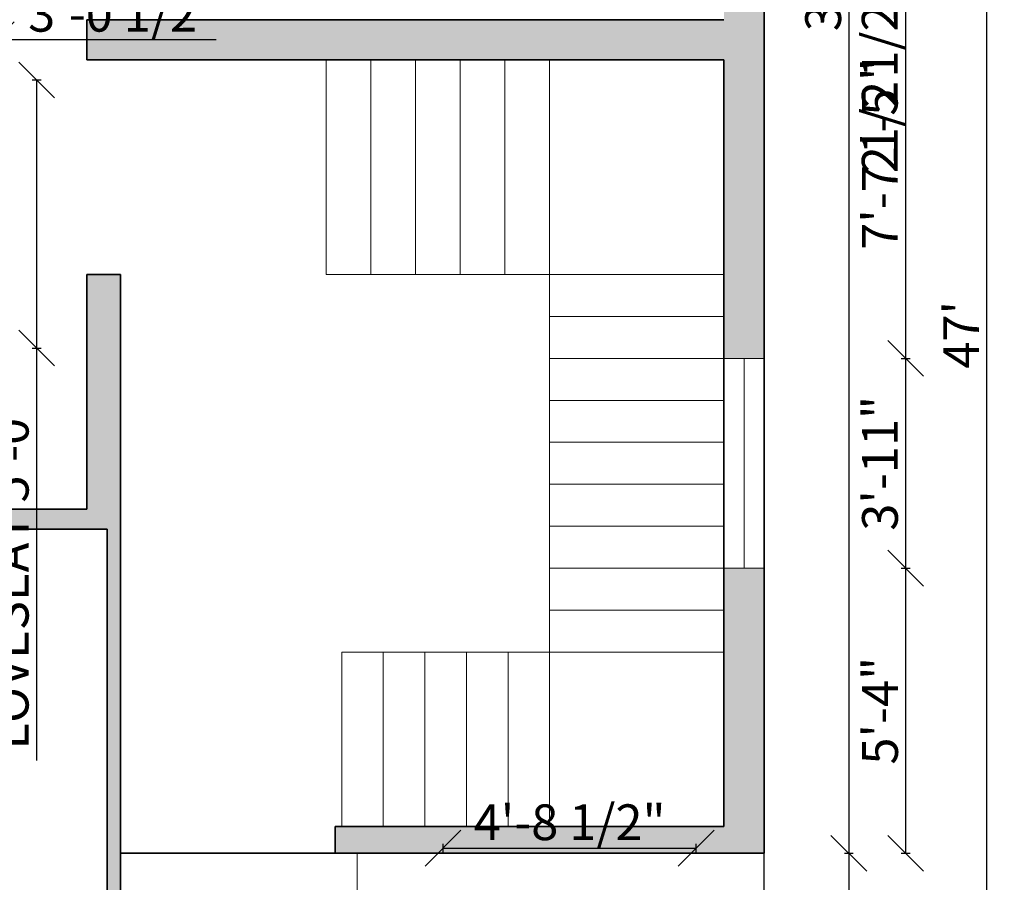
# Model space of a CAD drawing. Units: inches. Extents: x 2561 to 3163, y 493 to 1211.
# Tile 6 of 8: x 2943 to 3163, y 689 to 882. Entities that reach past the tile are written whole.
import ezdxf

# ---------------------------------------------------------------- set-up
doc = ezdxf.new("R2010")
doc.units = ezdxf.units.IN
for name, color, linetype, lineweight in [('A-ANNO-DIMS', 2, 'Continuous', 18), ('A-FLOR-STRS', 7, 'Continuous', 18), ('A-GLAZ', 4, 'Continuous', 18), ('A-SITE-PRKG', 8, 'Continuous', 25), ('A-WALL', 7, 'Continuous', 35), ('A-WALL-PATT', 24, 'Continuous', 13)]:
    doc.layers.add(name, color=color, linetype=linetype, lineweight=lineweight)
doc.styles.get("Standard").update_dxf_attribs({"font": 'arial.ttf'})
doc.dimstyles.new('ISO-25', dxfattribs={"dimtxt": 8, "dimasz": 8, "dimexe": 1, "dimexo": 1, "dimtad": 1, "dimlunit": 3, "dimtxsty": 'Standard', "dimblk": 'OBLIQUE', "dimcen": 2.5, "dimadec": 0, "dimazin": 0, "dimtfac": 1, "dimtmove": 0, "dimatfit": 3, "dimfxl": 1, "dimfxlon": 1, "dimarcsym": 0})

# ---------------------------------------------------------------- blocks, each defined once
blk = doc.blocks.new('_Oblique')
at = {"color": 0, "linetype": 'ByBlock', "lineweight": -2}
blk.add_line((-0.5, -0.5), (0.5, 0.5), dxfattribs=at)
blk = doc.blocks.new('*D10')
at = {"layer": 'A-ANNO-DIMS', "color": 0, "lineweight": -2, "transparency": 16777216}
for p, q in [((3127.21, 1093.07), (3129.21, 1093.07)), ((3128.21, 1093.07), (3128.21, 695.07)), ((3127.21, 695.07), (3129.21, 695.07))]:
    blk.add_line(p, q, dxfattribs=at)
at = {"layer": 'Defpoints', "color": 0, "transparency": 16777216}
for p in [(3109.27, 1093.07), (3109.27, 695.07), (3128.21, 695.07)]:
    blk.add_point(p, dxfattribs=at)
at = {"layer": 'A-ANNO-DIMS', "color": 0, "lineweight": -2, "transparency": 16777216, "xscale": 8, "yscale": 8, "zscale": 8}
for p, rotation in [((3128.21, 1093.07), 90), ((3128.21, 695.07), 270)]:
    blk.add_blockref('_Oblique', p, dxfattribs=dict(at, rotation=rotation))
at = {"layer": 'A-ANNO-DIMS', "color": 0, "transparency": 16777216, "insert": (3123.5, 894.07), "char_height": 8, "attachment_point": 5, "rotation": 90}
blk.add_mtext('33\'-2"', dxfattribs=at)
blk = doc.blocks.new('*D11')
at = {"layer": 'A-ANNO-DIMS', "color": 0, "lineweight": -2, "transparency": 16777216}
for p, q in [((3127.21, 695.07), (3129.21, 695.07)), ((3128.21, 695.07), (3128.21, 614.57)), ((3127.21, 614.57), (3129.21, 614.57))]:
    blk.add_line(p, q, dxfattribs=at)
at = {"layer": 'Defpoints', "color": 0, "transparency": 16777216}
for p in [(3109.27, 695.07), (2965.27, 614.57), (3128.21, 614.57)]:
    blk.add_point(p, dxfattribs=at)
at = {"layer": 'A-ANNO-DIMS', "color": 0, "lineweight": -2, "transparency": 16777216, "xscale": 8, "yscale": 8, "zscale": 8}
for p, rotation in [((3128.21, 695.07), 90), ((3128.21, 614.57), 270)]:
    blk.add_blockref('_Oblique', p, dxfattribs=dict(at, rotation=rotation))
at = {"layer": 'A-ANNO-DIMS', "color": 0, "transparency": 16777216, "insert": (3123.5, 654.82), "char_height": 8, "attachment_point": 5, "rotation": 90}
blk.add_mtext('6\'-8.5"', dxfattribs=at)
blk = doc.blocks.new('*D13')
at = {"layer": 'A-ANNO-DIMS', "color": 0, "lineweight": -2, "transparency": 16777216}
for p, q in [((3157.99, 1093.07), (3159.99, 1093.07)), ((3158.99, 1093.07), (3158.99, 529.07)), ((3157.99, 529.07), (3159.99, 529.07))]:
    blk.add_line(p, q, dxfattribs=at)
at = {"layer": 'Defpoints', "color": 0, "transparency": 16777216}
for p in [(3109.27, 1093.07), (3109.27, 529.07), (3158.99, 529.07)]:
    blk.add_point(p, dxfattribs=at)
at = {"layer": 'A-ANNO-DIMS', "color": 0, "lineweight": -2, "transparency": 16777216, "xscale": 8, "yscale": 8, "zscale": 8}
for p, rotation in [((3158.99, 1093.07), 90), ((3158.99, 529.07), 270)]:
    blk.add_blockref('_Oblique', p, dxfattribs=dict(at, rotation=rotation))
at = {"layer": 'A-ANNO-DIMS', "color": 0, "transparency": 16777216, "insert": (3154.37, 811.07), "char_height": 8, "attachment_point": 5, "rotation": 90}
blk.add_mtext("47'", dxfattribs=at)
blk = doc.blocks.new('*D17')
at = {"layer": 'A-ANNO-DIMS', "color": 0, "lineweight": -2, "transparency": 16777216}
for p, q in [((2571.63, 1093.07), (2569.63, 1093.07)), ((2570.63, 1093.07), (2570.63, 529.07)), ((2571.63, 529.07), (2569.63, 529.07))]:
    blk.add_line(p, q, dxfattribs=at)
at = {"layer": 'Defpoints', "color": 0, "transparency": 16777216}
for p in [(2629.27, 1093.07), (2570.63, 529.07), (3109.27, 529.07)]:
    blk.add_point(p, dxfattribs=at)
at = {"layer": 'A-ANNO-DIMS', "color": 0, "lineweight": -2, "transparency": 16777216, "xscale": 8, "yscale": 8, "zscale": 8}
for p, rotation in [((2570.63, 1093.07), 90), ((2570.63, 529.07), 270)]:
    blk.add_blockref('_Oblique', p, dxfattribs=dict(at, rotation=rotation))
at = {"layer": 'A-ANNO-DIMS', "color": 0, "transparency": 16777216, "insert": (2566, 811.07), "char_height": 8, "attachment_point": 5, "rotation": 90}
blk.add_mtext("47'", dxfattribs=at)
blk = doc.blocks.new('*D21')
at = {"layer": 'A-ANNO-DIMS', "color": 0, "lineweight": -2, "transparency": 16777216}
for p, q in [((3037.45, 695.2), (3037.45, 697.2)), ((3037.45, 696.2), (3094.06, 696.2)), ((3094.06, 695.2), (3094.06, 697.2))]:
    blk.add_line(p, q, dxfattribs=at)
at = {"layer": 'Defpoints', "color": 0, "transparency": 16777216}
for p in [(3094.06, 696.2), (3037.45, 676.33), (3094.06, 676.33)]:
    blk.add_point(p, dxfattribs=at)
at = {"layer": 'A-ANNO-DIMS', "color": 0, "lineweight": -2, "transparency": 16777216, "xscale": 8, "yscale": 8, "zscale": 8, "rotation": 180}
blk.add_blockref('_Oblique', (3037.45, 696.2), dxfattribs=at)
at = {"layer": 'A-ANNO-DIMS', "color": 0, "lineweight": -2, "transparency": 16777216, "xscale": 8, "yscale": 8, "zscale": 8}
blk.add_blockref('_Oblique', (3094.06, 696.2), dxfattribs=at)
at = {"layer": 'A-ANNO-DIMS', "color": 0, "transparency": 16777216, "insert": (3065.76, 700.97), "char_height": 8, "attachment_point": 5}
blk.add_mtext('4\'-8 1/2"', dxfattribs=at)
blk = doc.blocks.new('*D26')
at = {"layer": 'A-ANNO-DIMS', "color": 0, "lineweight": -2, "transparency": 16777216}
for p, q in [((2945.53, 868.1), (2947.53, 868.1)), ((2946.53, 868.1), (2946.53, 808.1)), ((2945.53, 808.1), (2947.53, 808.1)), ((2946.53, 808.1), (2946.53, 715.83))]:
    blk.add_line(p, q, dxfattribs=at)
at = {"layer": 'Defpoints', "color": 0, "transparency": 16777216}
for p in [(2937.53, 868.1), (2937.53, 808.1), (2946.53, 808.1)]:
    blk.add_point(p, dxfattribs=at)
at = {"layer": 'A-ANNO-DIMS', "color": 0, "lineweight": -2, "transparency": 16777216, "xscale": 8, "yscale": 8, "zscale": 8}
for p, rotation in [((2946.53, 868.1), 90), ((2946.53, 808.1), 270)]:
    blk.add_blockref('_Oblique', p, dxfattribs=dict(at, rotation=rotation))
at = {"layer": 'A-ANNO-DIMS', "color": 0, "transparency": 16777216, "insert": (2941.77, 757.96), "char_height": 8, "attachment_point": 5, "rotation": 90}
blk.add_mtext('LOVESEAT 5\'-0"', dxfattribs=at)
blk = doc.blocks.new('*D27')
at = {"layer": 'A-ANNO-DIMS', "color": 0, "lineweight": -2, "transparency": 16777216}
for p, q in [((2900.86, 876.1), (2900.86, 878.1)), ((2900.86, 877.1), (2937.53, 877.1)), ((2937.53, 876.1), (2937.53, 878.1)), ((2937.53, 877.1), (2986.68, 877.1))]:
    blk.add_line(p, q, dxfattribs=at)
at = {"layer": 'Defpoints', "color": 0, "transparency": 16777216}
for p in [(2937.53, 877.1), (2900.86, 868.1), (2937.53, 868.1)]:
    blk.add_point(p, dxfattribs=at)
at = {"layer": 'A-ANNO-DIMS', "color": 0, "lineweight": -2, "transparency": 16777216, "xscale": 8, "yscale": 8, "zscale": 8, "rotation": 180}
blk.add_blockref('_Oblique', (2900.86, 877.1), dxfattribs=at)
at = {"layer": 'A-ANNO-DIMS', "color": 0, "lineweight": -2, "transparency": 16777216, "xscale": 8, "yscale": 8, "zscale": 8}
blk.add_blockref('_Oblique', (2937.53, 877.1), dxfattribs=at)
at = {"layer": 'A-ANNO-DIMS', "color": 0, "transparency": 16777216, "insert": (2966.11, 881.86), "char_height": 8, "attachment_point": 5}
blk.add_mtext('3\'-0 1/2"', dxfattribs=at)
blk = doc.blocks.new('*D30')
at = {"layer": 'A-ANNO-DIMS', "color": 0, "lineweight": -2, "transparency": 16777216}
for p, q in [((2598.62, 740.07), (2596.62, 740.07)), ((2597.62, 740.07), (2597.62, 701.07)), ((2598.62, 701.07), (2596.62, 701.07))]:
    blk.add_line(p, q, dxfattribs=at)
at = {"layer": 'Defpoints', "color": 0, "transparency": 16777216}
for p in [(3014.77, 740.07), (2597.62, 701.07), (3014.77, 701.07)]:
    blk.add_point(p, dxfattribs=at)
at = {"layer": 'A-ANNO-DIMS', "color": 0, "lineweight": -2, "transparency": 16777216, "xscale": 8, "yscale": 8, "zscale": 8}
for p, rotation in [((2597.62, 740.07), 90), ((2597.62, 701.07), 270)]:
    blk.add_blockref('_Oblique', p, dxfattribs=dict(at, rotation=rotation))
at = {"layer": 'A-ANNO-DIMS', "color": 0, "transparency": 16777216, "insert": (2592.91, 720.57), "char_height": 8, "attachment_point": 5, "rotation": 90}
blk.add_mtext('3\'-3"', dxfattribs=at)
blk = doc.blocks.new('*D31')
at = {"layer": 'A-ANNO-DIMS', "color": 0, "lineweight": -2, "transparency": 16777216}
for p, q in [((2598.62, 872.57), (2596.62, 872.57)), ((2597.62, 824.57), (2597.62, 872.57)), ((2598.62, 824.57), (2596.62, 824.57))]:
    blk.add_line(p, q, dxfattribs=at)
at = {"layer": 'Defpoints', "color": 0, "transparency": 16777216}
for p in [(2597.62, 872.57), (3011.27, 872.57), (3011.27, 824.57)]:
    blk.add_point(p, dxfattribs=at)
at = {"layer": 'A-ANNO-DIMS', "color": 0, "lineweight": -2, "transparency": 16777216, "xscale": 8, "yscale": 8, "zscale": 8}
for p, rotation in [((2597.62, 872.57), 90), ((2597.62, 824.57), 270)]:
    blk.add_blockref('_Oblique', p, dxfattribs=dict(at, rotation=rotation))
at = {"layer": 'A-ANNO-DIMS', "color": 0, "transparency": 16777216, "insert": (2592.91, 848.57), "char_height": 8, "attachment_point": 5, "rotation": 90}
blk.add_mtext('4\'-0"', dxfattribs=at)
blk = doc.blocks.new('*D54')
at = {"layer": 'A-ANNO-DIMS', "color": 0, "lineweight": -2, "transparency": 16777216}
for p, q in [((3139.92, 927.07), (3141.92, 927.07)), ((3140.92, 927.07), (3140.92, 897.33)), ((3139.92, 897.33), (3141.92, 897.33)), ((3140.92, 897.33), (3140.92, 848.03))]:
    blk.add_line(p, q, dxfattribs=at)
at = {"layer": 'Defpoints', "color": 0, "transparency": 16777216}
for p in [(3109.27, 927.07), (3109.27, 897.33), (3140.92, 897.33)]:
    blk.add_point(p, dxfattribs=at)
at = {"layer": 'A-ANNO-DIMS', "color": 0, "lineweight": -2, "transparency": 16777216, "xscale": 8, "yscale": 8, "zscale": 8}
for p, rotation in [((3140.92, 927.07), 90), ((3140.92, 897.33), 270)]:
    blk.add_blockref('_Oblique', p, dxfattribs=dict(at, rotation=rotation))
at = {"layer": 'A-ANNO-DIMS', "color": 0, "transparency": 16777216, "insert": (3136.16, 868.68), "char_height": 8, "attachment_point": 5, "rotation": 90}
blk.add_mtext('2\'-5 1/2"', dxfattribs=at)
blk = doc.blocks.new('*D55')
at = {"layer": 'A-ANNO-DIMS', "color": 0, "lineweight": -2, "transparency": 16777216}
for p, q in [((3139.92, 897.33), (3141.92, 897.33)), ((3140.92, 897.33), (3140.92, 805.79)), ((3139.92, 805.79), (3141.92, 805.79))]:
    blk.add_line(p, q, dxfattribs=at)
at = {"layer": 'Defpoints', "color": 0, "transparency": 16777216}
for p in [(3109.27, 897.33), (3109.27, 805.79), (3140.92, 805.79)]:
    blk.add_point(p, dxfattribs=at)
at = {"layer": 'A-ANNO-DIMS', "color": 0, "lineweight": -2, "transparency": 16777216, "xscale": 8, "yscale": 8, "zscale": 8}
for p, rotation in [((3140.92, 897.33), 90), ((3140.92, 805.79), 270)]:
    blk.add_blockref('_Oblique', p, dxfattribs=dict(at, rotation=rotation))
at = {"layer": 'A-ANNO-DIMS', "color": 0, "transparency": 16777216, "insert": (3136.16, 851.56), "char_height": 8, "attachment_point": 5, "rotation": 90}
blk.add_mtext('7\'-7 1/2"', dxfattribs=at)
blk = doc.blocks.new('*D56')
at = {"layer": 'A-ANNO-DIMS', "color": 0, "lineweight": -2, "transparency": 16777216}
for p, q in [((3139.92, 805.79), (3141.92, 805.79)), ((3140.92, 805.79), (3140.92, 758.85)), ((3139.92, 758.85), (3141.92, 758.85))]:
    blk.add_line(p, q, dxfattribs=at)
at = {"layer": 'Defpoints', "color": 0, "transparency": 16777216}
for p in [(3109.27, 805.79), (3109.27, 758.85), (3140.92, 758.85)]:
    blk.add_point(p, dxfattribs=at)
at = {"layer": 'A-ANNO-DIMS', "color": 0, "lineweight": -2, "transparency": 16777216, "xscale": 8, "yscale": 8, "zscale": 8}
for p, rotation in [((3140.92, 805.79), 90), ((3140.92, 758.85), 270)]:
    blk.add_blockref('_Oblique', p, dxfattribs=dict(at, rotation=rotation))
at = {"layer": 'A-ANNO-DIMS', "color": 0, "transparency": 16777216, "insert": (3136.21, 782.32), "char_height": 8, "attachment_point": 5, "rotation": 90}
blk.add_mtext('3\'-11"', dxfattribs=at)
blk = doc.blocks.new('*D57')
at = {"layer": 'A-ANNO-DIMS', "color": 0, "lineweight": -2, "transparency": 16777216}
for p, q in [((3139.92, 758.85), (3141.92, 758.85)), ((3140.92, 758.85), (3140.92, 695.07)), ((3139.92, 695.07), (3141.92, 695.07))]:
    blk.add_line(p, q, dxfattribs=at)
at = {"layer": 'Defpoints', "color": 0, "transparency": 16777216}
for p in [(3109.27, 758.85), (3109.27, 695.07), (3140.92, 695.07)]:
    blk.add_point(p, dxfattribs=at)
at = {"layer": 'A-ANNO-DIMS', "color": 0, "lineweight": -2, "transparency": 16777216, "xscale": 8, "yscale": 8, "zscale": 8}
for p, rotation in [((3140.92, 758.85), 90), ((3140.92, 695.07), 270)]:
    blk.add_blockref('_Oblique', p, dxfattribs=dict(at, rotation=rotation))
at = {"layer": 'A-ANNO-DIMS', "color": 0, "transparency": 16777216, "insert": (3136.23, 726.96), "char_height": 8, "attachment_point": 5, "rotation": 90}
blk.add_mtext('5\'-4"', dxfattribs=at)

msp = doc.modelspace()

# ---------------------------------------------------------------- hatches: boundary and pattern name
at = {"layer": 'A-WALL-PATT'}
h = msp.add_hatch(color=256, dxfattribs=at)
h.dxf.hatch_style = 1
h.paths.add_polyline_path([(2665.022, 1093.069), (2629.274, 1093.069), (2629.274, 1056.034), (2638.274, 1056.034), (2638.274, 1084.069), (2665.022, 1084.069)])
h.paths.add_polyline_path([(2785.37, 1093.069), (2727.193, 1093.069), (2727.193, 1084.069), (2773.274, 1084.069), (2773.274, 940.069), (2762.774, 940.069), (2762.774, 935.569), (2777.774, 935.569), (2777.774, 971.569), (2825.774, 971.569), (2825.774, 935.569), (2921.774, 935.569), (2921.774, 940.069), (2830.274, 940.069), (2830.274, 976.069), (2777.774, 976.069), (2777.774, 1084.069), (2785.37, 1084.069)])
h.paths.add_polyline_path([(2856.568, 1093.069), (2816.168, 1093.069), (2816.168, 1084.069), (2825.774, 1084.069), (2825.774, 1008.069), (2830.274, 1008.069), (2830.274, 1084.069), (2856.568, 1084.069)], flags=17)
h.paths.add_polyline_path([(3006.866, 1093.069), (2929.24, 1093.069), (2929.24, 1084.069), (2962.274, 1084.069), (2962.274, 940.069), (2957.774, 940.069), (2957.774, 935.569), (2970.774, 935.569), (2970.774, 940.069), (2968.274, 940.069), (2968.274, 1084.069), (3006.866, 1084.069)])
h.paths.add_polyline_path([(3109.274, 1093.069), (3068.804, 1093.069), (3068.804, 1084.069), (3100.274, 1084.069), (3100.274, 1061.194), (3109.274, 1061.194)])
h.paths.add_polyline_path([(3109.274, 991.723), (3100.274, 991.723), (3100.274, 940.069), (3010.774, 940.069), (3010.774, 935.569), (3010.774, 911.569), (3015.274, 911.569), (3015.274, 935.569), (3100.274, 935.569), (3100.274, 927.07), (3109.274, 927.07)])
h.paths.add_polyline_path([(3109.274, 897.327), (3100.274, 897.327), (3100.274, 881.569), (2957.774, 881.569), (2957.774, 872.569), (3100.274, 872.569), (3100.274, 805.791), (3109.274, 805.791)])
h.paths.add_polyline_path([(2638.274, 982.372), (2629.274, 982.372), (2629.274, 927.027), (2638.274, 927.027), (2638.274, 935.569), (2722.274, 935.569), (2722.274, 919.569), (2726.774, 919.569), (2726.774, 940.069), (2638.274, 940.069)])
h.paths.add_polyline_path([(2638.274, 883.069), (2726.774, 883.069), (2726.774, 887.569), (2638.274, 887.569), (2638.274, 897.75), (2629.274, 897.75), (2629.274, 856.591), (2638.274, 856.591)])
h.paths.add_polyline_path([(2726.774, 851.069), (2722.274, 851.069), (2722.274, 772.069), (2638.274, 772.069), (2638.274, 802.178), (2629.274, 802.178), (2629.274, 725.136), (2638.274, 725.136), (2638.274, 767.569), (2726.774, 767.569)])
h.paths.add_polyline_path([(2638.274, 659.235), (2629.274, 659.235), (2629.274, 614.569), (2638.274, 614.569)])
h.paths.add_polyline_path([(2664.613, 623.569), (2638.274, 623.569), (2638.274, 614.569), (2664.613, 614.569)])
h.paths.add_polyline_path([(2787.908, 623.569), (2777.774, 623.569), (2777.774, 767.569), (2825.774, 767.569), (2825.774, 659.569), (2830.274, 659.569), (2830.274, 767.569), (2836.774, 767.569), (2836.774, 772.069), (2766.674, 772.069), (2766.674, 767.569), (2773.274, 767.569), (2773.274, 623.569), (2722.435, 623.569), (2722.435, 614.569), (2787.908, 614.569)])
h.paths.add_polyline_path([(2883.664, 623.569), (2867.474, 623.569), (2818.294, 623.569), (2818.294, 614.569), (2883.664, 614.569)])
h.paths.add_polyline_path([(2965.274, 772.069), (2872.774, 772.069), (2872.774, 767.569), (2962.274, 767.569), (2962.274, 623.569), (2936.565, 623.569), (2936.565, 614.569), (2965.274, 614.569)])
h.paths.add_polyline_path([(3109.274, 758.846), (3100.274, 758.846), (3100.274, 701.069), (3013.274, 701.069), (3013.274, 695.069), (3109.274, 695.069)])
h.paths.add_polyline_path([(2965.274, 824.569), (2957.774, 824.569), (2957.774, 772.069), (2965.274, 772.069)])

# ---------------------------------------------------------------- linework, layer by layer
at = {"layer": 'A-FLOR-STRS'}
for p, q in [((3011.274, 824.569), (3011.274, 872.569)), ((3021.274, 824.569), (3021.274, 872.569)), ((3031.274, 824.569), (3031.274, 872.569)), ((3041.274, 824.569), (3041.274, 872.569)), ((3051.274, 824.569), (3051.274, 872.569)), ((3061.274, 740.069), (3061.274, 872.569)), ((3011.274, 824.569), (3061.274, 824.569)), ((3061.274, 824.569), (3100.274, 824.569)), ((3061.274, 815.18), (3100.274, 815.18)), ((3061.274, 805.791), (3100.274, 805.791)), ((3061.274, 796.402), (3100.274, 796.402)), ((3061.274, 787.013), (3100.274, 787.013)), ((3061.274, 777.624), (3100.274, 777.624)), ((3061.274, 768.235), (3100.274, 768.235)), ((3061.274, 758.846), (3100.274, 758.846)), ((3061.274, 749.458), (3100.274, 749.458)), ((3014.774, 701.069), (3014.774, 740.069)), ((3014.774, 740.069), (3061.274, 740.069)), ((3024.074, 701.069), (3024.074, 740.069)), ((3033.374, 701.069), (3033.374, 740.069)), ((3042.674, 701.069), (3042.674, 740.069)), ((3051.974, 701.069), (3051.974, 740.069)), ((3061.274, 701.069), (3061.274, 740.069)), ((3100.274, 740.069), (3061.274, 740.069)), ((3018.195, 695.069), (3018.195, 677.069))]:
    msp.add_line(p, q, dxfattribs=at)
at = {"layer": 'A-GLAZ'}
for p, q in [((3100.274, 805.791), (3109.274, 805.791)), ((3100.274, 758.846), (3109.274, 758.846))]:
    msp.add_line(p, q, dxfattribs=at)
msp.add_lwpolyline([(3104.774, 758.846), (3104.774, 805.791)], dxfattribs=at)
at = {"layer": 'A-SITE-PRKG'}
msp.add_line((3109.274, 529.069), (3109.274, 695.069), dxfattribs=at)
at = {"layer": 'A-WALL'}
for p, q in [((3100.274, 881.569), (2957.774, 881.569)), ((2957.774, 872.569), (2957.774, 881.569)), ((3100.274, 872.569), (2957.774, 872.569)), ((3100.274, 701.069), (3100.274, 872.569)), ((2965.274, 824.569), (2957.774, 824.569)), ((2957.774, 824.569), (2957.774, 772.069)), ((2965.274, 772.069), (2965.274, 824.569)), ((2872.774, 772.069), (2957.774, 772.069)), ((2965.274, 614.569), (2965.274, 772.069)), ((2962.274, 767.569), (2872.774, 767.569)), ((2962.274, 623.569), (2962.274, 767.569)), ((3100.274, 701.069), (3013.274, 701.069)), ((3013.274, 701.069), (3013.274, 695.069)), ((3109.274, 695.069), (2965.274, 695.069))]:
    msp.add_line(p, q, dxfattribs=at)
msp.add_lwpolyline([(3109.274, 695.069), (3109.274, 1093.069), (2629.274, 1093.069), (2629.274, 614.569), (2965.274, 614.569)], dxfattribs=at)

# ---------------------------------------------------------------- dimensions: what is measured, and where the dimension line sits
at = {"layer": 'A-ANNO-DIMS'}
for base, p1, p2, angle, override, picture, middle in [((2570.627, 529.069), (2629.274, 1093.069), (3109.274, 529.069), 90, {"dimclrd": 0, "dimclre": 0, "dimclrt": 0}, '*D17', (2566.002, 811.069)), ((3128.213, 695.069), (3109.274, 1093.069), (3109.274, 695.069), 90, {"dimclrd": 0, "dimclre": 0, "dimclrt": 0}, '*D10', (3123.501, 894.069)), ((3158.992, 529.069), (3109.274, 1093.069), (3109.274, 529.069), 90, {"dimclrd": 0, "dimclre": 0, "dimclrt": 0}, '*D13', (3154.367, 811.069)), ((3140.924, 897.327), (3109.274, 927.07), (3109.274, 897.327), 270, {"dimdec": 1, "dimlfac": 1, "dimrnd": 0, "dimzin": 1, "dimdsep": 46, "dimlunit": 4, "dimfrac": 2}, '*D54', (3136.162, 868.681)), ((3140.924, 805.791), (3109.274, 897.327), (3109.274, 805.791), 270, {"dimdec": 1, "dimlfac": 1, "dimrnd": 0, "dimzin": 1, "dimdsep": 46, "dimlunit": 4, "dimfrac": 2}, '*D55', (3136.162, 851.559)), ((2597.624, 872.569), (3011.274, 824.569), (3011.274, 872.569), 90, {"dimdec": 1, "dimlfac": 1, "dimrnd": 0, "dimzin": 1, "dimdsep": 46, "dimlunit": 4, "dimfrac": 2}, '*D31', (2592.914, 848.569)), ((3140.924, 758.846), (3109.274, 805.791), (3109.274, 758.846), 270, {"dimdec": 1, "dimlfac": 1, "dimrnd": 0, "dimzin": 1, "dimdsep": 46, "dimlunit": 4, "dimfrac": 2}, '*D56', (3136.211, 782.319)), ((3140.924, 695.069), (3109.274, 758.846), (3109.274, 695.069), 270, {"dimdec": 1, "dimlfac": 1, "dimrnd": 0, "dimzin": 1, "dimdsep": 46, "dimlunit": 4, "dimfrac": 2}, '*D57', (3136.231, 726.958)), ((2597.624, 701.069), (3014.774, 740.069), (3014.774, 701.069), 90, {"dimdec": 1, "dimlfac": 1, "dimrnd": 0, "dimzin": 1, "dimdsep": 46, "dimlunit": 4, "dimfrac": 2}, '*D30', (2592.911, 720.569)), ((3128.213, 614.569), (3109.274, 695.069), (2965.274, 614.569), 90, {"dimclrd": 0, "dimclre": 0, "dimclrt": 0, "dimtmove": 1}, '*D11', (3123.503, 654.819))]:
    dim = msp.add_linear_dim(base=base, p1=p1, p2=p2, angle=angle, dimstyle='ISO-25', override=override, dxfattribs=at)
    dim.commit()
    dim.dimension.update_dxf_attribs({"geometry": picture, "text_midpoint": middle})
for base, p1, p2, picture, middle in [((2937.529, 877.099), (2900.863, 868.099), (2937.529, 868.099), '*D27', (2966.105, 881.863)), ((3094.064, 696.204), (3037.451, 676.333), (3094.064, 676.333), '*D21', (3065.757, 700.965))]:
    dim = msp.add_linear_dim(base=base, p1=p1, p2=p2, dimstyle='ISO-25', override={"dimdec": 1, "dimlfac": 1, "dimrnd": 0, "dimzin": 1, "dimdsep": 46, "dimlunit": 4, "dimfrac": 2}, dxfattribs=at)
    dim.commit()
    dim.dimension.update_dxf_attribs({"geometry": picture, "text_midpoint": middle})
dim = msp.add_linear_dim(base=(2946.529, 808.099), p1=(2937.529, 868.099), p2=(2937.529, 808.099), angle=270, text='LOVESEAT <>', dimstyle='ISO-25', override={"dimdec": 1, "dimlfac": 1, "dimrnd": 0, "dimzin": 1, "dimdsep": 46, "dimlunit": 4, "dimfrac": 2}, dxfattribs=at)
dim.commit()
dim.dimension.update_dxf_attribs({"geometry": '*D26', "text_midpoint": (2941.765, 757.962)})

doc.saveas('drawing.dxf')
